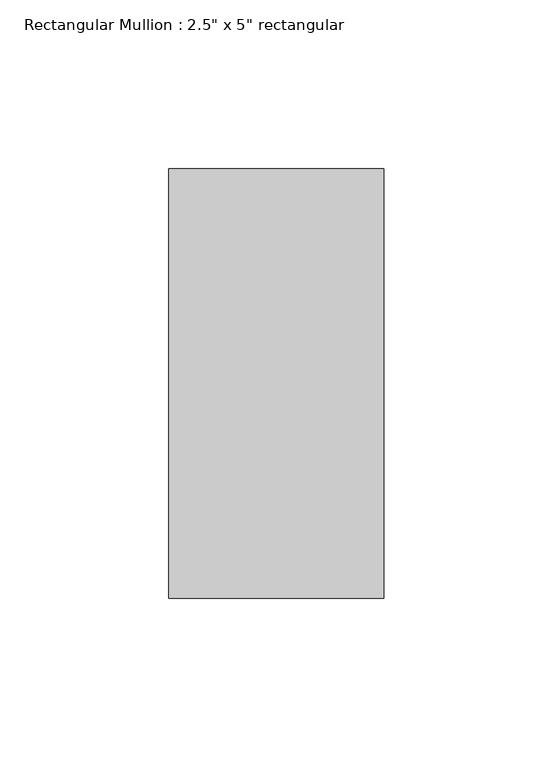
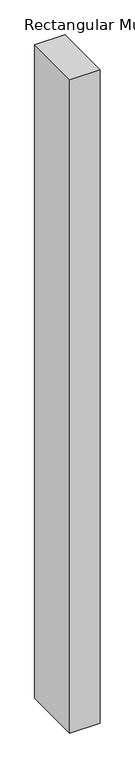
"""IFC4 building model written with IfcOpenShell, lengths in millimetres: member geometry."""

from ifc_helpers import new_model, si_unit, frame, origin, place, context, project, spatial, polyline, outline, extrude, source, transform, mapped, element, save


def member_77f995ea(model_context):
    return source(origin(), model_context, "Body", "SweptSolid", [
        extrude(outline(polyline([(0.0, 63.5), (0.0, -63.5), (-63.5, -63.5), (-63.5, 63.5), (0.0, 63.5)])), frame((0.0, 0.0, -1446.9814865), z_axis=(0.0, 0.0, 1.0), x_axis=(1.0, 0.0, 0.0)), (0.0, 0.0, 1.0), 1446.9814865),
    ])


if __name__ == "__main__":
    model = new_model("IFC4")
    model_context = context("Model", 3, world=origin())
    ifc_project = project(units=[si_unit("LENGTHUNIT", "METRE", prefix="MILLI")], contexts=[model_context])
    site = spatial("IfcSite", under=ifc_project)
    building = spatial("IfcBuilding", under=site)
    placement = place(None, origin())
    member_shape = member_77f995ea(model_context)
    element("IfcMember", 1, ObjectType="Rectangular Mullion : 2.5\" x 5\" rectangular", at=placement, inside=building, context=model_context, shape_type="MappedRepresentation", body=[
        mapped(member_shape, transform((0.0, 0.0, 0.0), x_axis=(1.0, 0.0, 0.0), y_axis=(0.0, 1.0, 0.0), z_axis=(0.0, 0.0, 1.0))),
    ])
    save(model, "model.ifc")

# Revit data of these elements
# Type "Rectangular Mullion : 2.5\" x 5\" rectangular"
#   built-in parameter 1007304 = 0.416667 (stored number, unit not read)
#   built-in parameter 1007301 = 0.104167 (stored number, unit not read)
#   built-in parameter 1007300 = 0.104167 (stored number, unit not read)
# Element 1 (IfcMember, "Rectangular Mullion : 2.5\" x 5\" rectangular")
#   Materials on its faces: "Aluminum"
# Materials
#   "Aluminum": class "Metal", colour RGB 247 247 247, transparency 0, Description = "Aluminum 6061", Cost = 0
